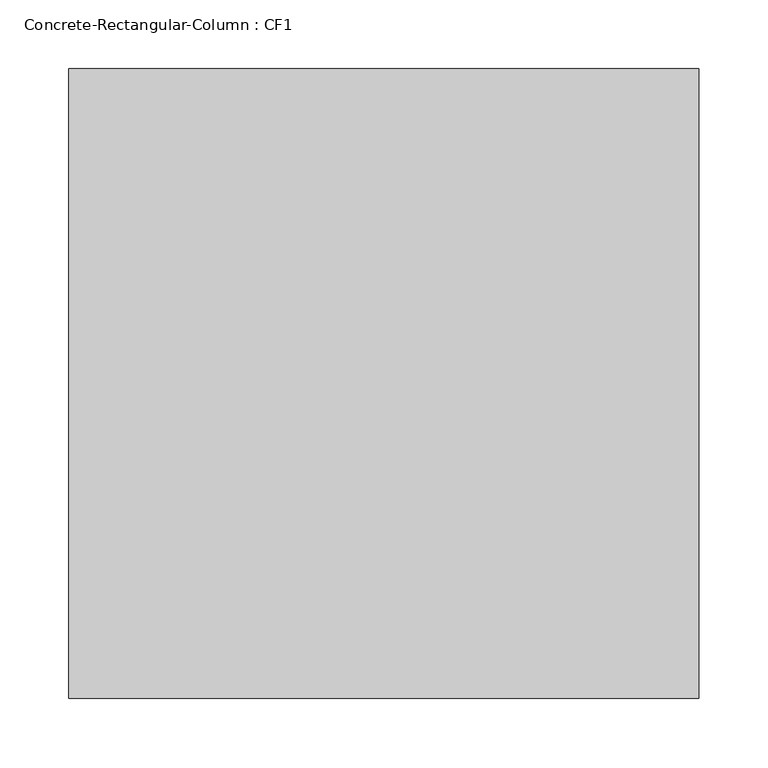
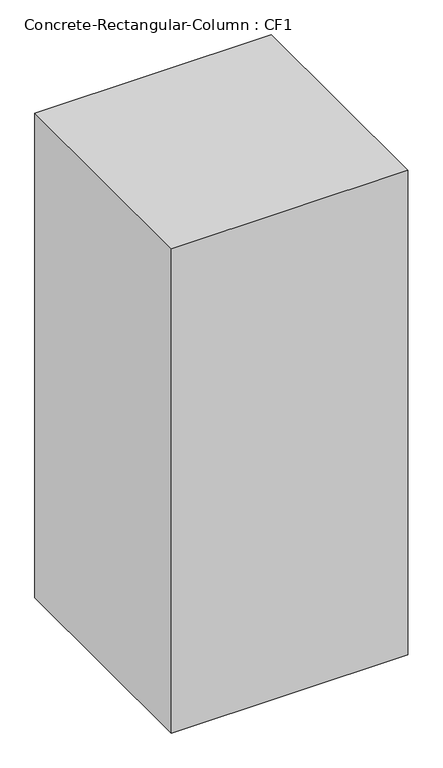
"""IFC4 building model written with IfcOpenShell, lengths in millimetres: column geometry, Concrete-Rectangular-Column : CF1."""

from ifc_helpers import new_model, si_unit, origin, origin_with_axes, place, context, project, spatial, polyline, outline, extrude, source, transform, mapped, element, save


def concrete_rectangular_column_cf1_9bf53746(model_context):
    return source(origin(), model_context, "Body", "SweptSolid", [
        extrude(outline(polyline([(228.6, 228.6), (228.6, -228.6), (-228.6, -228.6), (-228.6, 228.6), (228.6, 228.6)])), origin_with_axes(), (0.0, 0.0, 1.0), 990.6),
    ])


if __name__ == "__main__":
    model = new_model("IFC4")
    model_context = context("Model", 3, world=origin())
    ifc_project = project(units=[si_unit("LENGTHUNIT", "METRE", prefix="MILLI")], contexts=[model_context])
    site = spatial("IfcSite", under=ifc_project)
    building = spatial("IfcBuilding", under=site)
    placement = place(None, origin())
    concrete_rectangular_column_cf1_shape = concrete_rectangular_column_cf1_9bf53746(model_context)
    element("IfcColumn", 1, ObjectType="Concrete-Rectangular-Column : CF1", at=placement, inside=building, context=model_context, shape_type="MappedRepresentation", body=[
        mapped(concrete_rectangular_column_cf1_shape, transform((0.0, 0.0, 0.0), x_axis=(1.0, 0.0, 0.0), y_axis=(0.0, 1.0, 0.0), z_axis=(0.0, 0.0, 1.0))),
    ])
    save(model, "model.ifc")

# Revit data of these elements
# Type "Concrete-Rectangular-Column : CF1"
#   b = 457.2 mm
#   h = 457.2 mm
#   Structural Material [instance default] = Concrete, Cast-in-Place gray
# Element 1 (IfcColumn, "Concrete-Rectangular-Column : CF1")
#   Materials on its faces: "Concrete, Cast-in-Place gray"
# Materials
#   "Concrete, Cast-in-Place gray": class "Concrete", colour RGB 192 192 192, transparency 0, Description = "Cast-in-place concrete", Cost = 0
